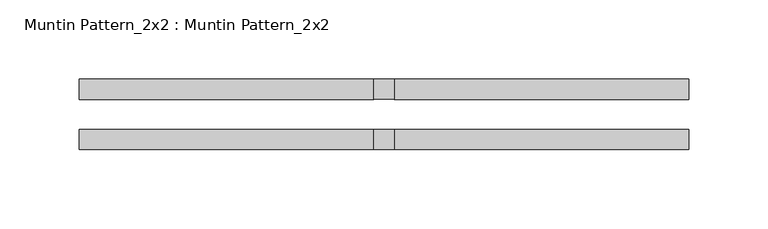
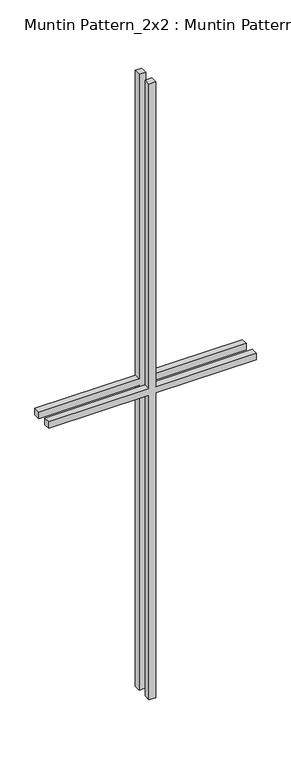
"""IFC4 building model written with IfcOpenShell, lengths in millimetres: proxy geometry, Muntin Pattern_2x2 : Muntin Pattern_2x2."""

from ifc_helpers import new_model, si_unit, frame, origin, place, context, project, spatial, polyline, outline, extrude, source, transform, mapped, element, save


def muntin_pattern_2x2_muntin_pattern_2x2_3dfd0a47(model_context):
    return source(origin(), model_context, "Body", "SweptSolid", [
        extrude(outline(polyline([(609.6, -6.35), (609.6, -192.0875), (596.9, -192.0875), (596.9, -6.35), (0.0, -6.35), (0.0, 6.35), (596.9, 6.35), (596.9, 192.0875), (609.6, 192.0875), (609.6, 6.35), (1206.5, 6.35), (1206.5, -6.35), (609.6, -6.35)])), frame((0.0, -22.225, 0.0), z_axis=(0.0, 1.0, 0.0), x_axis=(0.0, 0.0, 1.0)), (0.0, 0.0, 1.0), 12.7),
        extrude(outline(polyline([(609.6, -6.35), (609.6, -192.0875), (596.9, -192.0875), (596.9, -6.35), (0.0, -6.35), (0.0, 6.35), (596.9, 6.35), (596.9, 192.0875), (609.6, 192.0875), (609.6, 6.35), (1206.5, 6.35), (1206.5, -6.35), (609.6, -6.35)])), frame((0.0, 9.525, 0.0), z_axis=(0.0, 1.0, 0.0), x_axis=(0.0, 0.0, 1.0)), (0.0, 0.0, 1.0), 12.7),
    ])


if __name__ == "__main__":
    model = new_model("IFC4")
    model_context = context("Model", 3, world=origin())
    ifc_project = project(units=[si_unit("LENGTHUNIT", "METRE", prefix="MILLI")], contexts=[model_context])
    site = spatial("IfcSite", under=ifc_project)
    building = spatial("IfcBuilding", under=site)
    placement = place(None, origin())
    muntin_pattern_2x2_muntin_pattern_2x2_shape = muntin_pattern_2x2_muntin_pattern_2x2_3dfd0a47(model_context)
    element("IfcBuildingElementProxy", 1, Name="Muntin Pattern_2x2 : Muntin Pattern_2x2", ObjectType="Muntin Pattern_2x2 : Muntin Pattern_2x2", at=placement, inside=building, context=model_context, shape_type="MappedRepresentation", body=[
        mapped(muntin_pattern_2x2_muntin_pattern_2x2_shape, transform((0.0, 0.0, 0.0), x_axis=(1.0, 0.0, 0.0), y_axis=(0.0, 1.0, 0.0), z_axis=(0.0, 0.0, 1.0))),
    ])
    save(model, "model.ifc")

# Revit data of these elements
# Type "Muntin Pattern_2x2 : Muntin Pattern_2x2"
#   Width [instance default] = 4' - 0"
#   Thickness = 0' - 0 1/2"
#   Height [instance default] = 4' - 0"
#   Distance = 0' - 0 3/4"
#   Interior Material [instance default] = none
#   Exterior Material [instance default] = none
#   Default Elevation = 0
# Element 1 (IfcBuildingElementProxy, "Muntin Pattern_2x2 : Muntin Pattern_2x2")
#   Width = 1' - 3 1/8"
#   Height = 3' - 11 1/2"
#   Interior Material = Wood - Stained
#   Exterior Material = Clad - White
#   Materials on its faces: "Clad - White", "Wood - Stained"
# Materials
#   "Clad - White": class "Wood", colour RGB 242 242 238, transparency 0, Cost = 0
#   "Wood - Stained": class "Wood", colour RGB 224 178 126, transparency 0, Cost = 0
